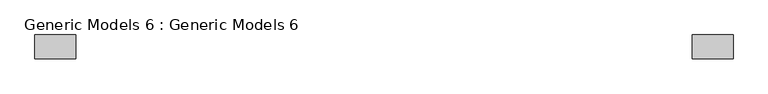
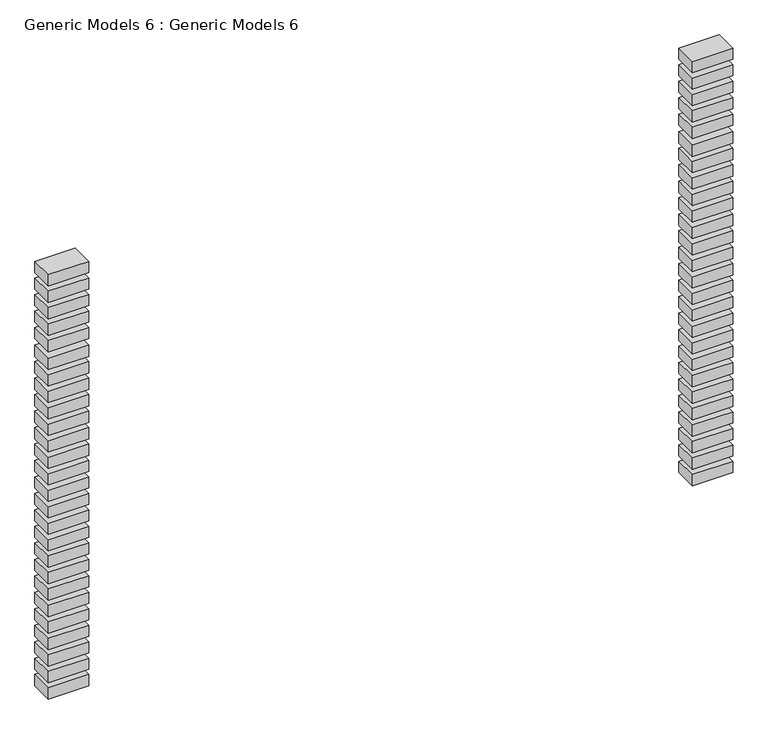
"""IFC4 building model written with IfcOpenShell, lengths in millimetres: proxy geometry, Generic Models 6 : Generic Models 6."""

from ifc_helpers import new_model, si_unit, frame, origin, place, context, project, spatial, polyline, outline, extrude, source, transform, mapped, element, save


def generic_models_6_generic_models_6_eab10de4(model_context):
    return source(origin(), model_context, "Body", "SweptSolid", [
        extrude(outline(polyline([(-11137.7236584, -13589.402305), (-11313.6293601, -13589.402305), (-11313.6293601, -13487.802305), (-11137.7236584, -13487.802305), (-11137.7236584, -13589.402305)])), frame((0.0, 0.0, 5594.5482366), z_axis=(0.0, 0.0, 1.0), x_axis=(1.0, 0.0, 0.0)), (0.0, 0.0, 1.0), 51.7732081),
        extrude(outline(polyline([(-11137.7236584, -13589.402305), (-11313.6293601, -13589.402305), (-11313.6293601, -13487.802305), (-11137.7236584, -13487.802305), (-11137.7236584, -13589.402305)])), frame((0.0, 0.0, 5518.3482366), z_axis=(0.0, 0.0, 1.0), x_axis=(1.0, 0.0, 0.0)), (0.0, 0.0, 1.0), 51.7732081),
        extrude(outline(polyline([(-11137.7236584, -13589.402305), (-11313.6293601, -13589.402305), (-11313.6293601, -13487.802305), (-11137.7236584, -13487.802305), (-11137.7236584, -13589.402305)])), frame((0.0, 0.0, 5442.1482366), z_axis=(0.0, 0.0, 1.0), x_axis=(1.0, 0.0, 0.0)), (0.0, 0.0, 1.0), 51.7732081),
        extrude(outline(polyline([(-11137.7236584, -13589.402305), (-11313.6293601, -13589.402305), (-11313.6293601, -13487.802305), (-11137.7236584, -13487.802305), (-11137.7236584, -13589.402305)])), frame((0.0, 0.0, 5365.9482366), z_axis=(0.0, 0.0, 1.0), x_axis=(1.0, 0.0, 0.0)), (0.0, 0.0, 1.0), 51.7732081),
        extrude(outline(polyline([(-11137.7236584, -13589.402305), (-11313.6293601, -13589.402305), (-11313.6293601, -13487.802305), (-11137.7236584, -13487.802305), (-11137.7236584, -13589.402305)])), frame((0.0, 0.0, 5289.7482366), z_axis=(0.0, 0.0, 1.0), x_axis=(1.0, 0.0, 0.0)), (0.0, 0.0, 1.0), 51.7732081),
        extrude(outline(polyline([(-11137.7236584, -13589.402305), (-11313.6293601, -13589.402305), (-11313.6293601, -13487.802305), (-11137.7236584, -13487.802305), (-11137.7236584, -13589.402305)])), frame((0.0, 0.0, 5207.1982366), z_axis=(0.0, 0.0, 1.0), x_axis=(1.0, 0.0, 0.0)), (0.0, 0.0, 1.0), 51.7732081),
        extrude(outline(polyline([(-11137.7236584, -13589.402305), (-11313.6293601, -13589.402305), (-11313.6293601, -13487.802305), (-11137.7236584, -13487.802305), (-11137.7236584, -13589.402305)])), frame((0.0, 0.0, 5130.9982366), z_axis=(0.0, 0.0, 1.0), x_axis=(1.0, 0.0, 0.0)), (0.0, 0.0, 1.0), 51.7732081),
        extrude(outline(polyline([(-11137.7236584, -13589.402305), (-11313.6293601, -13589.402305), (-11313.6293601, -13487.802305), (-11137.7236584, -13487.802305), (-11137.7236584, -13589.402305)])), frame((0.0, 0.0, 5054.7982366), z_axis=(0.0, 0.0, 1.0), x_axis=(1.0, 0.0, 0.0)), (0.0, 0.0, 1.0), 51.7732081),
        extrude(outline(polyline([(-11137.7236584, -13589.402305), (-11313.6293601, -13589.402305), (-11313.6293601, -13487.802305), (-11137.7236584, -13487.802305), (-11137.7236584, -13589.402305)])), frame((0.0, 0.0, 4978.5982366), z_axis=(0.0, 0.0, 1.0), x_axis=(1.0, 0.0, 0.0)), (0.0, 0.0, 1.0), 51.7732081),
        extrude(outline(polyline([(-11137.7236584, -13589.402305), (-11313.6293601, -13589.402305), (-11313.6293601, -13487.802305), (-11137.7236584, -13487.802305), (-11137.7236584, -13589.402305)])), frame((0.0, 0.0, 4902.3982366), z_axis=(0.0, 0.0, 1.0), x_axis=(1.0, 0.0, 0.0)), (0.0, 0.0, 1.0), 51.7732081),
        extrude(outline(polyline([(-11137.7236584, -13589.402305), (-11313.6293601, -13589.402305), (-11313.6293601, -13487.802305), (-11137.7236584, -13487.802305), (-11137.7236584, -13589.402305)])), frame((0.0, 0.0, 4826.1982366), z_axis=(0.0, 0.0, 1.0), x_axis=(1.0, 0.0, 0.0)), (0.0, 0.0, 1.0), 51.7732081),
        extrude(outline(polyline([(-11137.7236584, -13589.402305), (-11313.6293601, -13589.402305), (-11313.6293601, -13487.802305), (-11137.7236584, -13487.802305), (-11137.7236584, -13589.402305)])), frame((0.0, 0.0, 4749.9982366), z_axis=(0.0, 0.0, 1.0), x_axis=(1.0, 0.0, 0.0)), (0.0, 0.0, 1.0), 51.7732081),
        extrude(outline(polyline([(-11137.7236584, -13589.402305), (-11313.6293601, -13589.402305), (-11313.6293601, -13487.802305), (-11137.7236584, -13487.802305), (-11137.7236584, -13589.402305)])), frame((0.0, 0.0, 4673.7982366), z_axis=(0.0, 0.0, 1.0), x_axis=(1.0, 0.0, 0.0)), (0.0, 0.0, 1.0), 51.7732081),
        extrude(outline(polyline([(-11137.7236584, -13589.402305), (-11313.6293601, -13589.402305), (-11313.6293601, -13487.802305), (-11137.7236584, -13487.802305), (-11137.7236584, -13589.402305)])), frame((0.0, 0.0, 4597.5982366), z_axis=(0.0, 0.0, 1.0), x_axis=(1.0, 0.0, 0.0)), (0.0, 0.0, 1.0), 51.7732081),
        extrude(outline(polyline([(-11137.7236584, -13589.402305), (-11313.6293601, -13589.402305), (-11313.6293601, -13487.802305), (-11137.7236584, -13487.802305), (-11137.7236584, -13589.402305)])), frame((0.0, 0.0, 4521.3982366), z_axis=(0.0, 0.0, 1.0), x_axis=(1.0, 0.0, 0.0)), (0.0, 0.0, 1.0), 51.7732081),
        extrude(outline(polyline([(-11137.7236584, -13589.402305), (-11313.6293601, -13589.402305), (-11313.6293601, -13487.802305), (-11137.7236584, -13487.802305), (-11137.7236584, -13589.402305)])), frame((0.0, 0.0, 4445.1982366), z_axis=(0.0, 0.0, 1.0), x_axis=(1.0, 0.0, 0.0)), (0.0, 0.0, 1.0), 51.7732081),
        extrude(outline(polyline([(-11137.7236584, -13589.402305), (-11313.6293601, -13589.402305), (-11313.6293601, -13487.802305), (-11137.7236584, -13487.802305), (-11137.7236584, -13589.402305)])), frame((0.0, 0.0, 4368.9982366), z_axis=(0.0, 0.0, 1.0), x_axis=(1.0, 0.0, 0.0)), (0.0, 0.0, 1.0), 51.7732081),
        extrude(outline(polyline([(-11137.7236584, -13589.402305), (-11313.6293601, -13589.402305), (-11313.6293601, -13487.802305), (-11137.7236584, -13487.802305), (-11137.7236584, -13589.402305)])), frame((0.0, 0.0, 4292.7982366), z_axis=(0.0, 0.0, 1.0), x_axis=(1.0, 0.0, 0.0)), (0.0, 0.0, 1.0), 51.7732081),
        extrude(outline(polyline([(-11137.7236584, -13589.402305), (-11313.6293601, -13589.402305), (-11313.6293601, -13487.802305), (-11137.7236584, -13487.802305), (-11137.7236584, -13589.402305)])), frame((0.0, 0.0, 4216.5982366), z_axis=(0.0, 0.0, 1.0), x_axis=(1.0, 0.0, 0.0)), (0.0, 0.0, 1.0), 51.7732081),
        extrude(outline(polyline([(-11137.7236584, -13589.402305), (-11313.6293601, -13589.402305), (-11313.6293601, -13487.802305), (-11137.7236584, -13487.802305), (-11137.7236584, -13589.402305)])), frame((0.0, 0.0, 4140.3982366), z_axis=(0.0, 0.0, 1.0), x_axis=(1.0, 0.0, 0.0)), (0.0, 0.0, 1.0), 51.7732081),
        extrude(outline(polyline([(-11137.7236584, -13589.402305), (-11313.6293601, -13589.402305), (-11313.6293601, -13487.802305), (-11137.7236584, -13487.802305), (-11137.7236584, -13589.402305)])), frame((0.0, 0.0, 4064.1982366), z_axis=(0.0, 0.0, 1.0), x_axis=(1.0, 0.0, 0.0)), (0.0, 0.0, 1.0), 51.7732081),
        extrude(outline(polyline([(-11137.7236584, -13589.402305), (-11313.6293601, -13589.402305), (-11313.6293601, -13487.802305), (-11137.7236584, -13487.802305), (-11137.7236584, -13589.402305)])), frame((0.0, 0.0, 3987.9982366), z_axis=(0.0, 0.0, 1.0), x_axis=(1.0, 0.0, 0.0)), (0.0, 0.0, 1.0), 51.7732081),
        extrude(outline(polyline([(-11137.7236584, -13589.402305), (-11313.6293601, -13589.402305), (-11313.6293601, -13487.802305), (-11137.7236584, -13487.802305), (-11137.7236584, -13589.402305)])), frame((0.0, 0.0, 3911.7982366), z_axis=(0.0, 0.0, 1.0), x_axis=(1.0, 0.0, 0.0)), (0.0, 0.0, 1.0), 51.7732081),
        extrude(outline(polyline([(-11137.7236584, -13589.402305), (-11313.6293601, -13589.402305), (-11313.6293601, -13487.802305), (-11137.7236584, -13487.802305), (-11137.7236584, -13589.402305)])), frame((0.0, 0.0, 3835.5982366), z_axis=(0.0, 0.0, 1.0), x_axis=(1.0, 0.0, 0.0)), (0.0, 0.0, 1.0), 51.7732081),
        extrude(outline(polyline([(-11137.7236584, -13589.402305), (-11313.6293601, -13589.402305), (-11313.6293601, -13487.802305), (-11137.7236584, -13487.802305), (-11137.7236584, -13589.402305)])), frame((0.0, 0.0, 3759.3982366), z_axis=(0.0, 0.0, 1.0), x_axis=(1.0, 0.0, 0.0)), (0.0, 0.0, 1.0), 51.7732081),
        extrude(outline(polyline([(-11137.7236584, -13589.402305), (-11313.6293601, -13589.402305), (-11313.6293601, -13487.802305), (-11137.7236584, -13487.802305), (-11137.7236584, -13589.402305)])), frame((0.0, 0.0, 3683.1982366), z_axis=(0.0, 0.0, 1.0), x_axis=(1.0, 0.0, 0.0)), (0.0, 0.0, 1.0), 51.7732081),
        extrude(outline(polyline([(-8318.3236584, -13589.402305), (-8494.2293601, -13589.402305), (-8494.2293601, -13487.802305), (-8318.3236584, -13487.802305), (-8318.3236584, -13589.402305)])), frame((0.0, 0.0, 5594.5482366), z_axis=(0.0, 0.0, 1.0), x_axis=(1.0, 0.0, 0.0)), (0.0, 0.0, 1.0), 51.7732081),
        extrude(outline(polyline([(-8318.3236584, -13589.402305), (-8494.2293601, -13589.402305), (-8494.2293601, -13487.802305), (-8318.3236584, -13487.802305), (-8318.3236584, -13589.402305)])), frame((0.0, 0.0, 5518.3482366), z_axis=(0.0, 0.0, 1.0), x_axis=(1.0, 0.0, 0.0)), (0.0, 0.0, 1.0), 51.7732081),
        extrude(outline(polyline([(-8318.3236584, -13589.402305), (-8494.2293601, -13589.402305), (-8494.2293601, -13487.802305), (-8318.3236584, -13487.802305), (-8318.3236584, -13589.402305)])), frame((0.0, 0.0, 5442.1482366), z_axis=(0.0, 0.0, 1.0), x_axis=(1.0, 0.0, 0.0)), (0.0, 0.0, 1.0), 51.7732081),
        extrude(outline(polyline([(-8318.3236584, -13589.402305), (-8494.2293601, -13589.402305), (-8494.2293601, -13487.802305), (-8318.3236584, -13487.802305), (-8318.3236584, -13589.402305)])), frame((0.0, 0.0, 5365.9482366), z_axis=(0.0, 0.0, 1.0), x_axis=(1.0, 0.0, 0.0)), (0.0, 0.0, 1.0), 51.7732081),
        extrude(outline(polyline([(-8318.3236584, -13589.402305), (-8494.2293601, -13589.402305), (-8494.2293601, -13487.802305), (-8318.3236584, -13487.802305), (-8318.3236584, -13589.402305)])), frame((0.0, 0.0, 5289.7482366), z_axis=(0.0, 0.0, 1.0), x_axis=(1.0, 0.0, 0.0)), (0.0, 0.0, 1.0), 51.7732081),
        extrude(outline(polyline([(-8318.3236584, -13589.402305), (-8494.2293601, -13589.402305), (-8494.2293601, -13487.802305), (-8318.3236584, -13487.802305), (-8318.3236584, -13589.402305)])), frame((0.0, 0.0, 5207.1982366), z_axis=(0.0, 0.0, 1.0), x_axis=(1.0, 0.0, 0.0)), (0.0, 0.0, 1.0), 51.7732081),
        extrude(outline(polyline([(-8318.3236584, -13589.402305), (-8494.2293601, -13589.402305), (-8494.2293601, -13487.802305), (-8318.3236584, -13487.802305), (-8318.3236584, -13589.402305)])), frame((0.0, 0.0, 5130.9982366), z_axis=(0.0, 0.0, 1.0), x_axis=(1.0, 0.0, 0.0)), (0.0, 0.0, 1.0), 51.7732081),
        extrude(outline(polyline([(-8318.3236584, -13589.402305), (-8494.2293601, -13589.402305), (-8494.2293601, -13487.802305), (-8318.3236584, -13487.802305), (-8318.3236584, -13589.402305)])), frame((0.0, 0.0, 5054.7982366), z_axis=(0.0, 0.0, 1.0), x_axis=(1.0, 0.0, 0.0)), (0.0, 0.0, 1.0), 51.7732081),
        extrude(outline(polyline([(-8318.3236584, -13589.402305), (-8494.2293601, -13589.402305), (-8494.2293601, -13487.802305), (-8318.3236584, -13487.802305), (-8318.3236584, -13589.402305)])), frame((0.0, 0.0, 4978.5982366), z_axis=(0.0, 0.0, 1.0), x_axis=(1.0, 0.0, 0.0)), (0.0, 0.0, 1.0), 51.7732081),
        extrude(outline(polyline([(-8318.3236584, -13589.402305), (-8494.2293601, -13589.402305), (-8494.2293601, -13487.802305), (-8318.3236584, -13487.802305), (-8318.3236584, -13589.402305)])), frame((0.0, 0.0, 4902.3982366), z_axis=(0.0, 0.0, 1.0), x_axis=(1.0, 0.0, 0.0)), (0.0, 0.0, 1.0), 51.7732081),
        extrude(outline(polyline([(-8318.3236584, -13589.402305), (-8494.2293601, -13589.402305), (-8494.2293601, -13487.802305), (-8318.3236584, -13487.802305), (-8318.3236584, -13589.402305)])), frame((0.0, 0.0, 4826.1982366), z_axis=(0.0, 0.0, 1.0), x_axis=(1.0, 0.0, 0.0)), (0.0, 0.0, 1.0), 51.7732081),
        extrude(outline(polyline([(-8318.3236584, -13589.402305), (-8494.2293601, -13589.402305), (-8494.2293601, -13487.802305), (-8318.3236584, -13487.802305), (-8318.3236584, -13589.402305)])), frame((0.0, 0.0, 4749.9982366), z_axis=(0.0, 0.0, 1.0), x_axis=(1.0, 0.0, 0.0)), (0.0, 0.0, 1.0), 51.7732081),
        extrude(outline(polyline([(-8318.3236584, -13589.402305), (-8494.2293601, -13589.402305), (-8494.2293601, -13487.802305), (-8318.3236584, -13487.802305), (-8318.3236584, -13589.402305)])), frame((0.0, 0.0, 4673.7982366), z_axis=(0.0, 0.0, 1.0), x_axis=(1.0, 0.0, 0.0)), (0.0, 0.0, 1.0), 51.7732081),
        extrude(outline(polyline([(-8318.3236584, -13589.402305), (-8494.2293601, -13589.402305), (-8494.2293601, -13487.802305), (-8318.3236584, -13487.802305), (-8318.3236584, -13589.402305)])), frame((0.0, 0.0, 4597.5982366), z_axis=(0.0, 0.0, 1.0), x_axis=(1.0, 0.0, 0.0)), (0.0, 0.0, 1.0), 51.7732081),
        extrude(outline(polyline([(-8318.3236584, -13589.402305), (-8494.2293601, -13589.402305), (-8494.2293601, -13487.802305), (-8318.3236584, -13487.802305), (-8318.3236584, -13589.402305)])), frame((0.0, 0.0, 4521.3982366), z_axis=(0.0, 0.0, 1.0), x_axis=(1.0, 0.0, 0.0)), (0.0, 0.0, 1.0), 51.7732081),
        extrude(outline(polyline([(-8318.3236584, -13589.402305), (-8494.2293601, -13589.402305), (-8494.2293601, -13487.802305), (-8318.3236584, -13487.802305), (-8318.3236584, -13589.402305)])), frame((0.0, 0.0, 4445.1982366), z_axis=(0.0, 0.0, 1.0), x_axis=(1.0, 0.0, 0.0)), (0.0, 0.0, 1.0), 51.7732081),
        extrude(outline(polyline([(-8318.3236584, -13589.402305), (-8494.2293601, -13589.402305), (-8494.2293601, -13487.802305), (-8318.3236584, -13487.802305), (-8318.3236584, -13589.402305)])), frame((0.0, 0.0, 4368.9982366), z_axis=(0.0, 0.0, 1.0), x_axis=(1.0, 0.0, 0.0)), (0.0, 0.0, 1.0), 51.7732081),
        extrude(outline(polyline([(-8318.3236584, -13589.402305), (-8494.2293601, -13589.402305), (-8494.2293601, -13487.802305), (-8318.3236584, -13487.802305), (-8318.3236584, -13589.402305)])), frame((0.0, 0.0, 4292.7982366), z_axis=(0.0, 0.0, 1.0), x_axis=(1.0, 0.0, 0.0)), (0.0, 0.0, 1.0), 51.7732081),
        extrude(outline(polyline([(-8318.3236584, -13589.402305), (-8494.2293601, -13589.402305), (-8494.2293601, -13487.802305), (-8318.3236584, -13487.802305), (-8318.3236584, -13589.402305)])), frame((0.0, 0.0, 4216.5982366), z_axis=(0.0, 0.0, 1.0), x_axis=(1.0, 0.0, 0.0)), (0.0, 0.0, 1.0), 51.7732081),
        extrude(outline(polyline([(-8318.3236584, -13589.402305), (-8494.2293601, -13589.402305), (-8494.2293601, -13487.802305), (-8318.3236584, -13487.802305), (-8318.3236584, -13589.402305)])), frame((0.0, 0.0, 4140.3982366), z_axis=(0.0, 0.0, 1.0), x_axis=(1.0, 0.0, 0.0)), (0.0, 0.0, 1.0), 51.7732081),
        extrude(outline(polyline([(-8318.3236584, -13589.402305), (-8494.2293601, -13589.402305), (-8494.2293601, -13487.802305), (-8318.3236584, -13487.802305), (-8318.3236584, -13589.402305)])), frame((0.0, 0.0, 4064.1982366), z_axis=(0.0, 0.0, 1.0), x_axis=(1.0, 0.0, 0.0)), (0.0, 0.0, 1.0), 51.7732081),
        extrude(outline(polyline([(-8318.3236584, -13589.402305), (-8494.2293601, -13589.402305), (-8494.2293601, -13487.802305), (-8318.3236584, -13487.802305), (-8318.3236584, -13589.402305)])), frame((0.0, 0.0, 3987.9982366), z_axis=(0.0, 0.0, 1.0), x_axis=(1.0, 0.0, 0.0)), (0.0, 0.0, 1.0), 51.7732081),
        extrude(outline(polyline([(-8318.3236584, -13589.402305), (-8494.2293601, -13589.402305), (-8494.2293601, -13487.802305), (-8318.3236584, -13487.802305), (-8318.3236584, -13589.402305)])), frame((0.0, 0.0, 3911.7982366), z_axis=(0.0, 0.0, 1.0), x_axis=(1.0, 0.0, 0.0)), (0.0, 0.0, 1.0), 51.7732081),
        extrude(outline(polyline([(-8318.3236584, -13589.402305), (-8494.2293601, -13589.402305), (-8494.2293601, -13487.802305), (-8318.3236584, -13487.802305), (-8318.3236584, -13589.402305)])), frame((0.0, 0.0, 3835.5982366), z_axis=(0.0, 0.0, 1.0), x_axis=(1.0, 0.0, 0.0)), (0.0, 0.0, 1.0), 51.7732081),
        extrude(outline(polyline([(-8318.3236584, -13589.402305), (-8494.2293601, -13589.402305), (-8494.2293601, -13487.802305), (-8318.3236584, -13487.802305), (-8318.3236584, -13589.402305)])), frame((0.0, 0.0, 3759.3982366), z_axis=(0.0, 0.0, 1.0), x_axis=(1.0, 0.0, 0.0)), (0.0, 0.0, 1.0), 51.7732081),
        extrude(outline(polyline([(-8318.3236584, -13589.402305), (-8494.2293601, -13589.402305), (-8494.2293601, -13487.802305), (-8318.3236584, -13487.802305), (-8318.3236584, -13589.402305)])), frame((0.0, 0.0, 3683.1982366), z_axis=(0.0, 0.0, 1.0), x_axis=(1.0, 0.0, 0.0)), (0.0, 0.0, 1.0), 51.7732081),
    ])


if __name__ == "__main__":
    model = new_model("IFC4")
    model_context = context("Model", 3, world=origin())
    ifc_project = project(units=[si_unit("LENGTHUNIT", "METRE", prefix="MILLI")], contexts=[model_context])
    site = spatial("IfcSite", under=ifc_project)
    building = spatial("IfcBuilding", under=site)
    placement = place(None, origin())
    generic_models_6_generic_models_6_shape = generic_models_6_generic_models_6_eab10de4(model_context)
    element("IfcBuildingElementProxy", 1, Name="Generic Models 6 : Generic Models 6", ObjectType="Generic Models 6 : Generic Models 6", at=placement, inside=building, context=model_context, shape_type="MappedRepresentation", body=[
        mapped(generic_models_6_generic_models_6_shape, transform((0.0, 0.0, 0.0), x_axis=(1.0, 0.0, 0.0), y_axis=(0.0, 1.0, 0.0), z_axis=(0.0, 0.0, 1.0))),
    ])
    save(model, "model.ifc")

# Revit data of these elements
# Element 1 (IfcBuildingElementProxy, "Generic Models 6 : Generic Models 6")
#   Materials on its faces: "ACCENT BEIGE COLOUR"
# Materials
#   "ACCENT BEIGE COLOUR": class "Generic", colour RGB 120 120 120, transparency 0, Cost = 0
